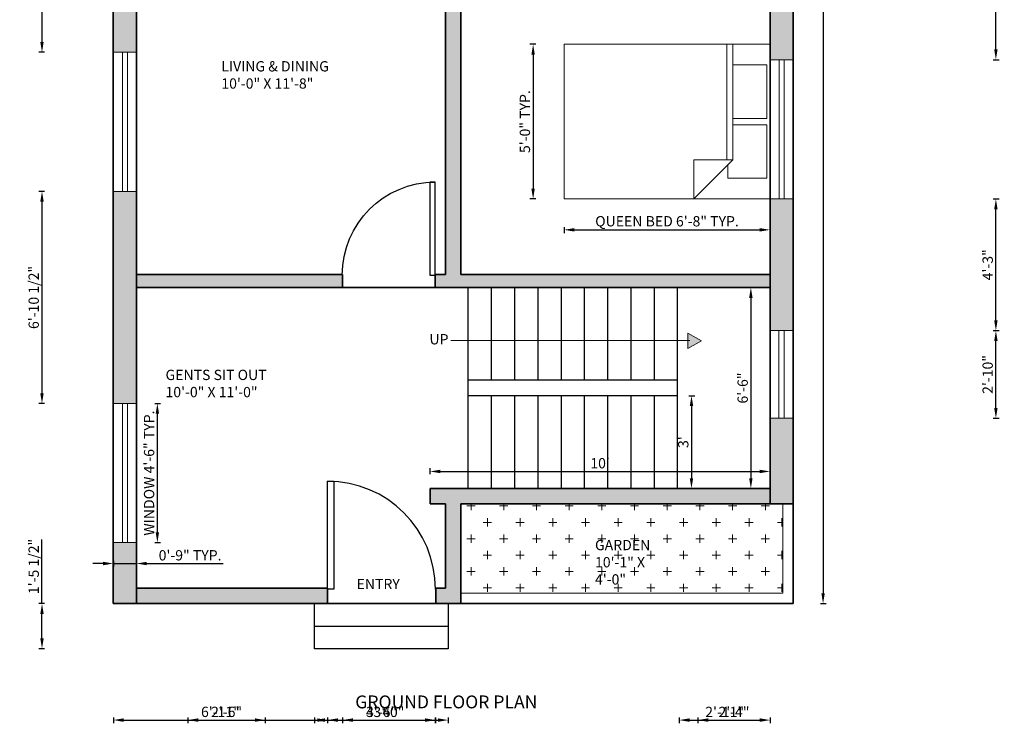
# Model space of a CAD drawing. Units: inches. Extents: x -34 to 348, y -513 to 46.
# Tile 1 of 2: x -34 to 348, y -513 to -240. Entities that reach past the tile are written whole.
import ezdxf

# ---------------------------------------------------------------- set-up
doc = ezdxf.new("R2010")
doc.units = ezdxf.units.IN
for name, color, linetype, lineweight in [('A-ANNO-DIMS', 2, 'Continuous', 18), ('A-ANNO-SYMB', 7, 'Continuous', 18), ('A-ANNO-TEXT', 7, 'Continuous', 18), ('A-AREA-IDEN', 7, 'Continuous', 18), ('A-DOOR', 4, 'Continuous', 25), ('A-FLOR-STRS', 7, 'Continuous', 25), ('A-FURN', 8, 'Continuous', 18), ('A-GLAZ', 6, 'Continuous', 18), ('A-WALL', 7, 'Continuous', 35), ('A-WALL-PATT', 251, 'Continuous', 13), ('L-PLNT', 3, 'Continuous', 18), ('L-PLNT-PATT', 3, 'Continuous', 13)]:
    doc.layers.add(name, color=color, linetype=linetype, lineweight=lineweight)
doc.styles.get("Standard").update_dxf_attribs({"font": 'arial.ttf'})
doc.dimstyles.new('ISO-25', dxfattribs={"dimtxt": 4, "dimasz": 4, "dimexe": 1.25, "dimexo": 0.625, "dimtad": 1, "dimlunit": 3, "dimtxsty": 'Standard', "dimcen": 2.5, "dimadec": 0, "dimazin": 0, "dimtfac": 1, "dimtmove": 0, "dimatfit": 3, "dimfxl": 1, "dimfxlon": 1, "dimarcsym": 0})

# ---------------------------------------------------------------- blocks, each defined once
blk = doc.blocks.new('*U4')
for p, q in [((0, 0), (0, -100)), ((750, 0), (750, -100))]:
    blk.add_line(p, q)
blk.add_lwpolyline([(0, 0), (0, 750), (43.75, 750), (43.75, 0)], close=True)
blk.add_arc((0, 0), 750, 0, 90)
blk = doc.blocks.new('Bed - Queen')
for p, q in [((0, -80.00003), (0, 0)), ((0, 0), (59.99999, 0)), ((59.99999, 0), (59.99999, -80.00003)), ((7.99999, -1.2), (28.79998, -1.2)), ((7.99999, -14.4), (7.99999, -1.2)), ((28.79998, -1.2), (28.79998, -14.4)), ((31.19999, -1.2), (51.99999, -1.2)), ((31.19999, -14.4), (31.19999, -1.2)), ((51.99999, -1.2), (51.99999, -16.4)), ((0, -14.4), (44.8, -14.4)), ((59.99999, -29.6), (44.8, -14.4)), ((44.8, -14.4), (44.8, -29.6)), ((44.8, -16.8), (0, -16.8)), ((51.99999, -16.4), (46.79936, -16.4)), ((44.8, -29.6), (59.99999, -29.6)), ((59.99999, -80.00003), (0, -80.00003))]:
    blk.add_line(p, q)
blk = doc.blocks.new('*D9')
at = {"layer": 'A-ANNO-DIMS', "color": 0, "lineweight": -2, "transparency": 16777216}
for p, q in [((225.63, -385.93), (227.88, -385.93)), ((226.63, -389.93), (226.63, -417.93)), ((225.63, -421.93), (227.88, -421.93))]:
    blk.add_line(p, q, dxfattribs=at)
at = {"layer": 'A-ANNO-DIMS', "color": 0, "transparency": 16777216}
for points in [[(225.96, -389.93), (227.3, -389.93), (226.63, -385.93)], [(225.96, -417.93), (227.3, -417.93), (226.63, -421.93)]]:
    blk.add_solid(points, dxfattribs=at)
at = {"layer": 'Defpoints', "color": 0, "transparency": 16777216}
for p in [(221.13, -385.93), (221.13, -421.93), (226.63, -421.93)]:
    blk.add_point(p, dxfattribs=at)
at = {"layer": 'A-ANNO-DIMS', "color": 0, "transparency": 16777216, "insert": (223.96, -403.93), "char_height": 4, "attachment_point": 5, "rotation": 90}
blk.add_mtext("3'", dxfattribs=at)
blk = doc.blocks.new('*D10')
at = {"layer": 'A-ANNO-DIMS', "color": 0, "lineweight": -2, "transparency": 16777216}
for p, q in [((125.13, -416.3), (125.13, -414.05)), ((129.13, -415.3), (253.13, -415.3)), ((257.13, -416.3), (257.13, -414.05))]:
    blk.add_line(p, q, dxfattribs=at)
at = {"layer": 'A-ANNO-DIMS', "color": 0, "transparency": 16777216}
for points in [[(129.13, -414.64), (129.13, -415.97), (125.13, -415.3)], [(253.13, -414.64), (253.13, -415.97), (257.13, -415.3)]]:
    blk.add_solid(points, dxfattribs=at)
at = {"layer": 'Defpoints', "color": 0, "transparency": 16777216}
for p in [(257.13, -415.3), (125.13, -421.93), (257.13, -421.93)]:
    blk.add_point(p, dxfattribs=at)
at = {"layer": 'A-ANNO-DIMS', "color": 0, "transparency": 16777216, "insert": (191.13, -412.63), "char_height": 4, "attachment_point": 5}
blk.add_mtext("10'", dxfattribs=at)
blk = doc.blocks.new('*D11')
at = {"layer": 'A-ANNO-DIMS', "color": 0, "lineweight": -2, "transparency": 16777216}
for p, q in [((250.69, -343.93), (248.44, -343.93)), ((249.69, -347.93), (249.69, -417.93)), ((250.69, -421.93), (248.44, -421.93))]:
    blk.add_line(p, q, dxfattribs=at)
at = {"layer": 'A-ANNO-DIMS', "color": 0, "transparency": 16777216}
for points in [[(249.02, -347.93), (250.35, -347.93), (249.69, -343.93)], [(249.02, -417.93), (250.35, -417.93), (249.69, -421.93)]]:
    blk.add_solid(points, dxfattribs=at)
at = {"layer": 'Defpoints', "color": 0, "transparency": 16777216}
for p in [(257.13, -343.93), (249.69, -421.93), (257.13, -421.93)]:
    blk.add_point(p, dxfattribs=at)
at = {"layer": 'A-ANNO-DIMS', "color": 0, "transparency": 16777216, "insert": (247.02, -382.93), "char_height": 4, "attachment_point": 5, "rotation": 90}
blk.add_mtext('6\'-6"', dxfattribs=at)
blk = doc.blocks.new('*D13')
at = {"layer": 'A-ANNO-DIMS', "color": 0, "lineweight": -2, "transparency": 16777216}
for p, q in [((276.72, 13.4), (278.97, 13.4)), ((277.72, 9.4), (277.72, -462.6)), ((276.72, -466.6), (278.97, -466.6))]:
    blk.add_line(p, q, dxfattribs=at)
at = {"layer": 'A-ANNO-DIMS', "color": 0, "transparency": 16777216}
for points in [[(277.06, 9.4), (278.39, 9.4), (277.72, 13.4)], [(277.06, -462.6), (278.39, -462.6), (277.72, -466.6)]]:
    blk.add_solid(points, dxfattribs=at)
at = {"layer": 'Defpoints', "color": 0, "transparency": 16777216}
for p in [(266.13, 13.4), (266.13, -466.6), (277.72, -466.6)]:
    blk.add_point(p, dxfattribs=at)
at = {"layer": 'A-ANNO-DIMS', "color": 0, "transparency": 16777216, "insert": (275.05, -226.6), "char_height": 4, "attachment_point": 5, "rotation": 90}
blk.add_mtext("40'", dxfattribs=at)
blk = doc.blocks.new('WIN-54IN')
for p, q in [((3.5, 54), (3.5, 0)), ((5.5, 54), (5.5, 0))]:
    blk.add_line(p, q)
blk.add_lwpolyline([(0, 54), (9, 54), (9, 0), (0, 0)], close=True)
blk = doc.blocks.new('*D16')
at = {"layer": 'A-ANNO-DIMS', "color": 0, "lineweight": -2, "transparency": 16777216}
for p, q in [((18.23, -388.94), (20.48, -388.94)), ((19.23, -438.94), (19.23, -392.94)), ((18.23, -442.94), (20.48, -442.94))]:
    blk.add_line(p, q, dxfattribs=at)
at = {"layer": 'A-ANNO-DIMS', "color": 0, "transparency": 16777216}
for points in [[(18.56, -392.94), (19.89, -392.94), (19.23, -388.94)], [(18.56, -438.94), (19.89, -438.94), (19.23, -442.94)]]:
    blk.add_solid(points, dxfattribs=at)
at = {"layer": 'Defpoints', "color": 0, "transparency": 16777216}
for p in [(11.13, -388.94), (19.23, -388.94), (11.13, -442.94)]:
    blk.add_point(p, dxfattribs=at)
at = {"layer": 'A-ANNO-DIMS', "color": 0, "transparency": 16777216, "insert": (16.53, -415.94), "char_height": 4, "attachment_point": 5, "rotation": 90}
blk.add_mtext('WINDOW 4\'-6" TYP.', dxfattribs=at)
blk = doc.blocks.new('*D17')
at = {"layer": 'A-ANNO-DIMS', "color": 0, "lineweight": -2, "transparency": 16777216}
for p, q in [((-1.87, -451.04), (-5.87, -451.04)), ((2.13, -450.04), (2.13, -452.29)), ((2.13, -451.04), (11.13, -451.04)), ((11.13, -450.04), (11.13, -452.29)), ((15.13, -451.04), (44.76, -451.04))]:
    blk.add_line(p, q, dxfattribs=at)
at = {"layer": 'A-ANNO-DIMS', "color": 0, "transparency": 16777216}
for points in [[(-1.87, -450.37), (-1.87, -451.71), (2.13, -451.04)], [(15.13, -450.37), (15.13, -451.71), (11.13, -451.04)]]:
    blk.add_solid(points, dxfattribs=at)
at = {"layer": 'Defpoints', "color": 0, "transparency": 16777216}
for p in [(2.13, -442.94), (11.13, -442.94), (11.13, -451.04)]:
    blk.add_point(p, dxfattribs=at)
at = {"layer": 'A-ANNO-DIMS', "color": 0, "transparency": 16777216, "insert": (31.94, -448.37), "char_height": 4, "attachment_point": 5}
blk.add_mtext('0\'-9" TYP.', dxfattribs=at)
blk = doc.blocks.new('*D20')
at = {"layer": 'A-ANNO-DIMS', "color": 0, "lineweight": -2, "transparency": 16777216}
for p, q in [((177.13, -320.53), (177.13, -322.78)), ((257.13, -320.53), (257.13, -322.78)), ((181.13, -321.53), (253.13, -321.53))]:
    blk.add_line(p, q, dxfattribs=at)
at = {"layer": 'A-ANNO-DIMS', "color": 0, "transparency": 16777216}
for points in [[(181.13, -320.87), (181.13, -322.2), (177.13, -321.53)], [(253.13, -320.87), (253.13, -322.2), (257.13, -321.53)]]:
    blk.add_solid(points, dxfattribs=at)
at = {"layer": 'Defpoints', "color": 0, "transparency": 16777216}
for p in [(177.13, -309.53), (257.13, -309.53), (257.13, -321.53)]:
    blk.add_point(p, dxfattribs=at)
at = {"layer": 'A-ANNO-DIMS', "color": 0, "transparency": 16777216, "insert": (217.13, -318.72), "char_height": 4, "attachment_point": 5}
blk.add_mtext('QUEEN BED 6\'-8" TYP.', dxfattribs=at)
blk = doc.blocks.new('*D21')
at = {"layer": 'A-ANNO-DIMS', "color": 0, "lineweight": -2, "transparency": 16777216}
for p, q in [((166.13, -249.53), (163.88, -249.53)), ((165.13, -253.53), (165.13, -305.53)), ((166.13, -309.53), (163.88, -309.53))]:
    blk.add_line(p, q, dxfattribs=at)
at = {"layer": 'A-ANNO-DIMS', "color": 0, "transparency": 16777216}
for points in [[(164.46, -253.53), (165.79, -253.53), (165.13, -249.53)], [(164.46, -305.53), (165.79, -305.53), (165.13, -309.53)]]:
    blk.add_solid(points, dxfattribs=at)
at = {"layer": 'Defpoints', "color": 0, "transparency": 16777216}
for p in [(177.13, -249.53), (165.13, -309.53), (177.13, -309.53)]:
    blk.add_point(p, dxfattribs=at)
at = {"layer": 'A-ANNO-DIMS', "color": 0, "transparency": 16777216, "insert": (162.46, -279.53), "char_height": 4, "attachment_point": 5, "rotation": 90}
blk.add_mtext('5\'-0" TYP.', dxfattribs=at)
blk = doc.blocks.new('*D28')
at = {"layer": 'A-ANNO-DIMS', "color": 0, "lineweight": -2, "transparency": 16777216}
for p, q in [((80.3, -510.8), (80.3, -513.05)), ((84.3, -511.8), (128.17, -511.8)), ((132.17, -510.8), (132.17, -513.05))]:
    blk.add_line(p, q, dxfattribs=at)
at = {"layer": 'A-ANNO-DIMS', "color": 0, "transparency": 16777216}
for points in [[(84.3, -511.13), (84.3, -512.47), (80.3, -511.8)], [(128.17, -511.13), (128.17, -512.47), (132.17, -511.8)]]:
    blk.add_solid(points, dxfattribs=at)
at = {"layer": 'Defpoints', "color": 0, "transparency": 16777216}
for p in [(80.3, -484.1), (132.17, -484.1), (132.17, -511.8)]:
    blk.add_point(p, dxfattribs=at)
at = {"layer": 'A-ANNO-DIMS', "color": 0, "transparency": 16777216, "insert": (106.23, -509.17), "char_height": 4, "attachment_point": 5}
blk.add_mtext('4\'-4"', dxfattribs=at)
blk = doc.blocks.new('*D29')
at = {"layer": 'A-ANNO-DIMS', "color": 0, "lineweight": -2, "transparency": 16777216}
for p, q in [((-25.57, -466.6), (-25.57, -441.77)), ((-24.57, -466.6), (-26.82, -466.6)), ((-25.57, -480.1), (-25.57, -470.6)), ((-24.57, -484.1), (-26.82, -484.1))]:
    blk.add_line(p, q, dxfattribs=at)
at = {"layer": 'A-ANNO-DIMS', "color": 0, "transparency": 16777216}
for points in [[(-26.24, -470.6), (-24.91, -470.6), (-25.57, -466.6)], [(-26.24, -480.1), (-24.91, -480.1), (-25.57, -484.1)]]:
    blk.add_solid(points, dxfattribs=at)
at = {"layer": 'Defpoints', "color": 0, "transparency": 16777216}
for p in [(-25.57, -466.6), (80.3, -466.6), (80.3, -484.1)]:
    blk.add_point(p, dxfattribs=at)
at = {"layer": 'A-ANNO-DIMS', "color": 0, "transparency": 16777216, "insert": (-28.27, -452.18), "char_height": 4, "attachment_point": 5, "rotation": 90}
blk.add_mtext('1\'-5 1/2"', dxfattribs=at)
blk = doc.blocks.new('*D30')
at = {"layer": 'A-ANNO-DIMS', "color": 0, "lineweight": -2, "transparency": 16777216}
for p, q in [((85.32, -510.8), (85.32, -513.05)), ((89.32, -511.8), (123.24, -511.8)), ((127.24, -510.8), (127.24, -513.05))]:
    blk.add_line(p, q, dxfattribs=at)
at = {"layer": 'A-ANNO-DIMS', "color": 0, "transparency": 16777216}
for points in [[(89.32, -511.13), (89.32, -512.47), (85.32, -511.8)], [(123.24, -511.13), (123.24, -512.47), (127.24, -511.8)]]:
    blk.add_solid(points, dxfattribs=at)
at = {"layer": 'Defpoints', "color": 0, "transparency": 16777216}
for p in [(85.32, -466.6), (127.24, -466.6), (127.24, -511.8)]:
    blk.add_point(p, dxfattribs=at)
at = {"layer": 'A-ANNO-DIMS', "color": 0, "transparency": 16777216, "insert": (106.28, -509.13), "char_height": 4, "attachment_point": 5}
blk.add_mtext('3\'-6"', dxfattribs=at)
blk = doc.blocks.new('*D31')
at = {"layer": 'A-ANNO-DIMS', "color": 0, "lineweight": -2, "transparency": 16777216}
for p, q in [((2.13, -510.8), (2.13, -513.05)), ((6.13, -511.8), (81.32, -511.8)), ((85.32, -510.8), (85.32, -513.05))]:
    blk.add_line(p, q, dxfattribs=at)
at = {"layer": 'A-ANNO-DIMS', "color": 0, "transparency": 16777216}
for points in [[(6.13, -511.13), (6.13, -512.47), (2.13, -511.8)], [(81.32, -511.13), (81.32, -512.47), (85.32, -511.8)]]:
    blk.add_solid(points, dxfattribs=at)
at = {"layer": 'Defpoints', "color": 0, "transparency": 16777216}
for p in [(2.13, -466.6), (85.32, -466.6), (85.32, -511.8)]:
    blk.add_point(p, dxfattribs=at)
at = {"layer": 'A-ANNO-DIMS', "color": 0, "transparency": 16777216, "insert": (43.72, -509.13), "char_height": 4, "attachment_point": 5}
blk.add_mtext('6\'-11"', dxfattribs=at)
blk = doc.blocks.new('*D32')
at = {"layer": 'A-ANNO-DIMS', "color": 0, "lineweight": -2, "transparency": 16777216}
for p, q in [((91.13, -510.8), (91.13, -513.05)), ((95.13, -511.8), (123.13, -511.8)), ((127.13, -510.8), (127.13, -513.05))]:
    blk.add_line(p, q, dxfattribs=at)
at = {"layer": 'A-ANNO-DIMS', "color": 0, "transparency": 16777216}
for points in [[(95.13, -511.13), (95.13, -512.47), (91.13, -511.8)], [(123.13, -511.13), (123.13, -512.47), (127.13, -511.8)]]:
    blk.add_solid(points, dxfattribs=at)
at = {"layer": 'Defpoints', "color": 0, "transparency": 16777216}
for p in [(91.13, -343.93), (127.13, -343.93), (127.13, -511.8)]:
    blk.add_point(p, dxfattribs=at)
at = {"layer": 'A-ANNO-DIMS', "color": 0, "transparency": 16777216, "insert": (109.13, -509.13), "char_height": 4, "attachment_point": 5}
blk.add_mtext('3\'-0"', dxfattribs=at)
blk = doc.blocks.new('*D33')
at = {"layer": 'A-ANNO-DIMS', "color": 0, "lineweight": -2, "transparency": 16777216}
for p, q in [((31.1, -510.8), (31.1, -513.05)), ((35.1, -511.8), (57.12, -511.8)), ((61.12, -510.8), (61.12, -513.05))]:
    blk.add_line(p, q, dxfattribs=at)
at = {"layer": 'A-ANNO-DIMS', "color": 0, "transparency": 16777216}
for points in [[(35.1, -511.13), (35.1, -512.47), (31.1, -511.8)], [(57.12, -511.13), (57.12, -512.47), (61.12, -511.8)]]:
    blk.add_solid(points, dxfattribs=at)
at = {"layer": 'Defpoints', "color": 0, "transparency": 16777216}
for p in [(31.1, -137.74), (61.12, -137.74), (61.12, -511.8)]:
    blk.add_point(p, dxfattribs=at)
at = {"layer": 'A-ANNO-DIMS', "color": 0, "transparency": 16777216, "insert": (46.11, -509.13), "char_height": 4, "attachment_point": 5}
blk.add_mtext('2\'-6"', dxfattribs=at)
blk = doc.blocks.new('*D41')
at = {"layer": 'A-ANNO-DIMS', "color": 0, "lineweight": -2, "transparency": 16777216}
for p, q in [((-24.57, -190.01), (-26.82, -190.01)), ((-25.57, -194.01), (-25.57, -248.61)), ((-24.57, -252.61), (-26.82, -252.61))]:
    blk.add_line(p, q, dxfattribs=at)
at = {"layer": 'A-ANNO-DIMS', "color": 0, "transparency": 16777216}
for points in [[(-26.24, -194.01), (-24.91, -194.01), (-25.57, -190.01)], [(-26.24, -248.61), (-24.91, -248.61), (-25.57, -252.61)]]:
    blk.add_solid(points, dxfattribs=at)
at = {"layer": 'Defpoints', "color": 0, "transparency": 16777216}
for p in [(2.13, -190.01), (-25.57, -252.61), (2.13, -252.61)]:
    blk.add_point(p, dxfattribs=at)
at = {"layer": 'A-ANNO-DIMS', "color": 0, "transparency": 16777216, "insert": (-28.27, -221.31), "char_height": 4, "attachment_point": 5, "rotation": 90}
blk.add_mtext('5\'-2 1/2"', dxfattribs=at)
blk = doc.blocks.new('*D42')
at = {"layer": 'A-ANNO-DIMS', "color": 0, "lineweight": -2, "transparency": 16777216}
for p, q in [((-24.57, -306.61), (-26.82, -306.61)), ((-25.57, -310.61), (-25.57, -384.94)), ((-24.57, -388.94), (-26.82, -388.94))]:
    blk.add_line(p, q, dxfattribs=at)
at = {"layer": 'A-ANNO-DIMS', "color": 0, "transparency": 16777216}
for points in [[(-26.24, -310.61), (-24.91, -310.61), (-25.57, -306.61)], [(-26.24, -384.94), (-24.91, -384.94), (-25.57, -388.94)]]:
    blk.add_solid(points, dxfattribs=at)
at = {"layer": 'Defpoints', "color": 0, "transparency": 16777216}
for p in [(2.13, -306.61), (-25.57, -388.94), (2.13, -388.94)]:
    blk.add_point(p, dxfattribs=at)
at = {"layer": 'A-ANNO-DIMS', "color": 0, "transparency": 16777216, "insert": (-28.27, -347.78), "char_height": 4, "attachment_point": 5, "rotation": 90}
blk.add_mtext('6\'-10 1/2"', dxfattribs=at)
blk = doc.blocks.new('*D45')
at = {"layer": 'A-ANNO-DIMS', "color": 0, "lineweight": -2, "transparency": 16777216}
for p, q in [((343.83, -190.01), (346.08, -190.01)), ((344.83, -251.53), (344.83, -194.01)), ((343.83, -255.53), (346.08, -255.53))]:
    blk.add_line(p, q, dxfattribs=at)
at = {"layer": 'A-ANNO-DIMS', "color": 0, "transparency": 16777216}
for points in [[(344.16, -194.01), (345.49, -194.01), (344.83, -190.01)], [(344.16, -251.53), (345.49, -251.53), (344.83, -255.53)]]:
    blk.add_solid(points, dxfattribs=at)
at = {"layer": 'Defpoints', "color": 0, "transparency": 16777216}
for p in [(266.13, -190.01), (344.83, -190.01), (266.13, -255.53)]:
    blk.add_point(p, dxfattribs=at)
at = {"layer": 'A-ANNO-DIMS', "color": 0, "transparency": 16777216, "insert": (342.13, -222.77), "char_height": 4, "attachment_point": 5, "rotation": 90}
blk.add_mtext('5\'-5 1/2"', dxfattribs=at)
blk = doc.blocks.new('*D46')
at = {"layer": 'A-ANNO-DIMS', "color": 0, "lineweight": -2, "transparency": 16777216}
for p, q in [((343.83, -309.53), (346.08, -309.53)), ((344.83, -356.66), (344.83, -313.53)), ((343.83, -360.66), (346.08, -360.66))]:
    blk.add_line(p, q, dxfattribs=at)
at = {"layer": 'A-ANNO-DIMS', "color": 0, "transparency": 16777216}
for points in [[(344.16, -313.53), (345.49, -313.53), (344.83, -309.53)], [(344.16, -356.66), (345.49, -356.66), (344.83, -360.66)]]:
    blk.add_solid(points, dxfattribs=at)
at = {"layer": 'Defpoints', "color": 0, "transparency": 16777216}
for p in [(266.13, -309.53), (344.83, -309.53), (266.11, -360.66)]:
    blk.add_point(p, dxfattribs=at)
at = {"layer": 'A-ANNO-DIMS', "color": 0, "transparency": 16777216, "insert": (342.16, -335.1), "char_height": 4, "attachment_point": 5, "rotation": 90}
blk.add_mtext('4\'-3"', dxfattribs=at)
blk = doc.blocks.new('*D47')
at = {"layer": 'A-ANNO-DIMS', "color": 0, "lineweight": -2, "transparency": 16777216}
for p, q in [((343.83, -360.66), (346.08, -360.66)), ((344.83, -390.66), (344.83, -364.66)), ((343.83, -394.66), (346.08, -394.66))]:
    blk.add_line(p, q, dxfattribs=at)
at = {"layer": 'A-ANNO-DIMS', "color": 0, "transparency": 16777216}
for points in [[(344.16, -364.66), (345.49, -364.66), (344.83, -360.66)], [(344.16, -390.66), (345.49, -390.66), (344.83, -394.66)]]:
    blk.add_solid(points, dxfattribs=at)
at = {"layer": 'Defpoints', "color": 0, "transparency": 16777216}
for p in [(266.11, -360.66), (344.83, -360.66), (266.11, -394.66)]:
    blk.add_point(p, dxfattribs=at)
at = {"layer": 'A-ANNO-DIMS', "color": 0, "transparency": 16777216, "insert": (342.16, -377.66), "char_height": 4, "attachment_point": 5, "rotation": 90}
blk.add_mtext('2\'-10"', dxfattribs=at)
blk = doc.blocks.new('*D49')
at = {"layer": 'A-ANNO-DIMS', "color": 0, "lineweight": -2, "transparency": 16777216}
for p, q in [((229.13, -510.8), (229.13, -513.05)), ((233.13, -511.8), (253.13, -511.8)), ((257.13, -510.8), (257.13, -513.05))]:
    blk.add_line(p, q, dxfattribs=at)
at = {"layer": 'A-ANNO-DIMS', "color": 0, "transparency": 16777216}
for points in [[(233.13, -511.13), (233.13, -512.47), (229.13, -511.8)], [(253.13, -511.13), (253.13, -512.47), (257.13, -511.8)]]:
    blk.add_solid(points, dxfattribs=at)
at = {"layer": 'Defpoints', "color": 0, "transparency": 16777216}
for p in [(229.13, -167.74), (257.13, -178.24), (257.13, -511.8)]:
    blk.add_point(p, dxfattribs=at)
at = {"layer": 'A-ANNO-DIMS', "color": 0, "transparency": 16777216, "insert": (243.13, -509.17), "char_height": 4, "attachment_point": 5}
blk.add_mtext('2\'-4"', dxfattribs=at)
blk = doc.blocks.new('*D50')
at = {"layer": 'A-ANNO-DIMS', "color": 0, "lineweight": -2, "transparency": 16777216}
for p, q in [((221.89, -510.8), (221.89, -513.05)), ((225.89, -511.8), (253.13, -511.8)), ((257.13, -510.8), (257.13, -513.05))]:
    blk.add_line(p, q, dxfattribs=at)
at = {"layer": 'A-ANNO-DIMS', "color": 0, "transparency": 16777216}
for points in [[(225.89, -511.13), (225.89, -512.47), (221.89, -511.8)], [(253.13, -511.13), (253.13, -512.47), (257.13, -511.8)]]:
    blk.add_solid(points, dxfattribs=at)
at = {"layer": 'Defpoints', "color": 0, "transparency": 16777216}
for p in [(221.89, 4.4), (257.13, 4.4), (257.13, -511.8)]:
    blk.add_point(p, dxfattribs=at)
at = {"layer": 'A-ANNO-DIMS', "color": 0, "transparency": 16777216, "insert": (239.51, -509.17), "char_height": 4, "attachment_point": 5}
blk.add_mtext('2\'-11"', dxfattribs=at)
blk = doc.blocks.new('*D51')
at = {"layer": 'A-ANNO-DIMS', "color": 0, "lineweight": -2, "transparency": 16777216}
for p, q in [((221.13, 40.1), (221.13, 42.35)), ((257.13, 40.1), (257.13, 42.35)), ((225.13, 41.1), (253.13, 41.1))]:
    blk.add_line(p, q, dxfattribs=at)
at = {"layer": 'A-ANNO-DIMS', "color": 0, "transparency": 16777216}
for points in [[(225.13, 41.77), (225.13, 40.44), (221.13, 41.1)], [(253.13, 41.77), (253.13, 40.44), (257.13, 41.1)]]:
    blk.add_solid(points, dxfattribs=at)
at = {"layer": 'Defpoints', "color": 0, "transparency": 16777216}
for p in [(257.13, 41.1), (221.13, -343.93), (257.13, -343.93)]:
    blk.add_point(p, dxfattribs=at)
at = {"layer": 'A-ANNO-DIMS', "color": 0, "transparency": 16777216, "insert": (239.13, 43.77), "char_height": 4, "attachment_point": 5}
blk.add_mtext('3\'-0"', dxfattribs=at)
blk = doc.blocks.new('*D53')
at = {"layer": 'A-ANNO-DIMS', "color": 0, "lineweight": -2, "transparency": 16777216}
for p, q in [((212.09, 40.1), (212.09, 42.35)), ((221.13, 40.1), (221.13, 42.35)), ((208.09, 41.1), (204.09, 41.1)), ((212.09, 41.1), (221.13, 41.1)), ((225.13, 41.1), (241.01, 41.1))]:
    blk.add_line(p, q, dxfattribs=at)
at = {"layer": 'A-ANNO-DIMS', "color": 0, "transparency": 16777216}
for points in [[(208.09, 41.77), (208.09, 40.44), (212.09, 41.1)], [(225.13, 41.77), (225.13, 40.44), (221.13, 41.1)]]:
    blk.add_solid(points, dxfattribs=at)
at = {"layer": 'Defpoints', "color": 0, "transparency": 16777216}
for p in [(221.13, 41.1), (212.09, -343.93), (221.13, -343.93)]:
    blk.add_point(p, dxfattribs=at)
at = {"layer": 'A-ANNO-DIMS', "color": 0, "transparency": 16777216, "insert": (235.07, 43.77), "char_height": 4, "attachment_point": 5}
blk.add_mtext('0\'-9"', dxfattribs=at)

msp = doc.modelspace()

# ---------------------------------------------------------------- hatches: boundary and pattern name
at = {"layer": 'A-ANNO-SYMB'}
h = msp.add_hatch(color=256, dxfattribs=at)
h.dxf.hatch_style = 1
h.paths.add_polyline_path([(225.262, -361.599), (225.262, -367.599), (230.46, -364.602)])
at = {"layer": 'A-WALL-PATT'}
h = msp.add_hatch(color=256, dxfattribs=at)
h.dxf.hatch_style = 1
h.paths.add_polyline_path([(109.341, 13.405), (2.127, 13.405), (2.127, -25.971), (11.127, -25.971), (11.127, 4.405), (109.341, 4.405)])
h.paths.add_polyline_path([(266.127, 13.405), (127.341, 13.405), (127.341, 4.405), (131.127, 4.405), (137.127, 4.405), (257.127, 4.405), (257.127, -24.182), (266.127, -24.182)])
h.paths.add_polyline_path([(11.127, -79.971), (2.127, -79.971), (2.127, -172.013), (11.127, -172.013)])
h.paths.add_polyline_path([(65.127, -127.595), (11.127, -127.595), (11.127, -133.595), (59.127, -133.595), (59.127, -137.743), (61.124, -137.743), (65.127, -137.743), (65.127, -133.595)])
h.paths.add_polyline_path([(65.127, -167.764), (61.124, -167.764, -0.0092932), (60.008, -167.743), (59.127, -167.743), (59.127, -193.595), (11.127, -193.595), (11.127, -199.595), (59.127, -199.595), (65.127, -199.595)])
h.paths.add_polyline_path([(11.127, -190.013), (2.127, -190.013), (2.127, -252.614), (11.127, -252.614)])
h.paths.add_polyline_path([(11.127, -306.614), (2.127, -306.614), (2.127, -388.939), (11.127, -388.939)])
h.paths.add_polyline_path([(85.316, -461.006), (85.316, -460.595), (11.127, -460.595), (11.127, -466.595), (85.316, -466.595)])
h.paths.add_polyline_path([(11.127, -442.939), (2.127, -442.939), (2.127, -466.595), (11.127, -466.595)])
h.paths.add_polyline_path([(137.127, -427.93), (257.127, -427.93), (257.127, -421.93), (131.127, -421.93), (125.127, -421.93), (125.127, -427.93), (131.127, -427.93), (131.127, -460.595), (127.316, -460.595), (127.316, -466.595), (132.166, -466.595), (137.127, -466.595)])
h.paths.add_polyline_path([(266.127, -394.659), (257.127, -394.659), (257.127, -421.93), (257.127, -427.93), (266.127, -427.93)])
h.paths.add_polyline_path([(266.127, -309.532), (257.127, -309.532), (257.127, -343.93), (257.127, -360.659), (266.127, -360.659)])
h.paths.add_polyline_path([(257.127, -338.93), (137.127, -338.93), (137.127, -199.595), (141.127, -199.595), (141.127, -193.595), (131.127, -193.595), (131.127, -338.93), (127.127, -338.93), (127.127, -339.114), (127.127, -343.93), (137.127, -343.93), (257.127, -343.93)])
h.paths.add_polyline_path([(91.006, -338.93), (11.127, -338.93), (11.127, -343.93), (91.006, -343.93)])
h.paths.add_polyline_path([(266.127, -190.013), (257.127, -190.013), (257.127, -255.532), (266.127, -255.532)])
h.paths.add_polyline_path([(257.127, -193.595), (185.127, -193.595), (185.127, -167.989), (179.127, -167.989), (179.127, -193.595), (177.136, -193.595), (177.136, -198.391, -0.0057168), (177.127, -199.214), (177.127, -199.595), (179.127, -199.595), (185.127, -199.595), (257.127, -199.595)])
h.paths.add_polyline_path([(266.127, -78.182), (257.127, -78.182), (257.127, -172.013), (266.127, -172.013)])
h.paths.add_polyline_path([(257.127, -127.595), (177.127, -127.595), (177.127, -133.595), (179.127, -133.595), (179.127, -137.989), (183.118, -137.989), (185.127, -137.989), (185.127, -133.595), (257.127, -133.595)])
h.paths.add_polyline_path([(137.127, 4.405), (131.127, 4.405), (131.127, -127.595), (127.127, -127.595), (127.127, -133.595), (131.127, -133.595), (137.127, -133.595), (141.127, -133.595), (141.127, -128.797), (141.127, -127.595), (137.127, -127.595)])
at = {"layer": 'L-PLNT-PATT'}
h = msp.add_hatch(dxfattribs=at)
h.set_pattern_fill('CROSS', color=256)
h.set_pattern_definition([(0, (-419.374, -35.0104), (6.35, 6.35), [3.175, -9.525]), (90, (-417.7867, -36.598), (-6.35, 6.35), [3.175, -9.525])])
h.paths.add_polyline_path([(262.127, -427.93), (137.127, -427.93), (137.127, -462.595), (262.127, -462.595)])

# ---------------------------------------------------------------- linework, layer by layer
at = {"layer": 'A-ANNO-SYMB'}
msp.add_line((133.139, -364.529), (226.006, -364.529), dxfattribs=at)
msp.add_lwpolyline([(225.262, -361.599), (225.262, -367.599), (230.46, -364.602)], close=True, dxfattribs=at)
at = {"layer": 'A-FLOR-STRS'}
for p, q in [((139.832, -343.93), (139.832, -421.93)), ((139.832, -343.93), (139.832, -379.93)), ((148.865, -343.93), (148.865, -379.93)), ((157.897, -343.93), (157.897, -379.93)), ((166.93, -343.93), (166.93, -379.93)), ((175.963, -343.93), (175.963, -379.93)), ((184.996, -343.93), (184.996, -379.93)), ((194.028, -343.93), (194.028, -379.93)), ((203.061, -343.93), (203.061, -379.93)), ((212.094, -343.93), (212.094, -379.93)), ((221.127, -343.93), (221.127, -379.93)), ((221.127, -379.93), (139.832, -379.93)), ((221.127, -379.93), (221.127, -385.93)), ((221.127, -385.93), (139.832, -385.93)), ((139.832, -385.93), (139.832, -421.93)), ((148.865, -385.93), (148.865, -421.93)), ((157.897, -385.93), (157.897, -421.93)), ((166.93, -385.93), (166.93, -421.93)), ((175.963, -385.93), (175.963, -421.93)), ((184.996, -385.93), (184.996, -421.93)), ((194.028, -385.93), (194.028, -421.93)), ((203.061, -385.93), (203.061, -421.93)), ((212.094, -385.93), (212.094, -421.93)), ((221.127, -385.93), (221.127, -421.93)), ((80.303, -475.348), (132.166, -475.348))]:
    msp.add_line(p, q, dxfattribs=at)
msp.add_lwpolyline([(80.303, -466.595), (132.166, -466.595), (132.166, -484.1), (80.303, -484.1)], close=True, dxfattribs=at)
at = {"layer": 'A-GLAZ'}
for p, q in [((5.627, -252.614), (5.627, -306.614)), ((7.627, -252.614), (7.627, -306.614)), ((260.606, -360.659), (260.606, -394.659)), ((262.606, -360.659), (262.606, -394.659))]:
    msp.add_line(p, q, dxfattribs=at)
for points in [[(2.127, -252.614), (11.127, -252.614), (11.127, -306.614), (2.127, -306.614)], [(257.106, -360.659), (266.106, -360.659), (266.106, -394.659), (257.106, -394.659)]]:
    msp.add_lwpolyline(points, close=True, dxfattribs=at)
at = {"layer": 'A-WALL'}
for p, q in [((2.127, -466.595), (2.127, 13.405)), ((266.127, 13.405), (266.127, -427.93)), ((11.127, -466.595), (11.127, 4.405)), ((257.127, 4.405), (257.127, -343.93)), ((131.127, -338.93), (131.127, -193.595)), ((137.127, -338.93), (137.127, -199.595)), ((91.127, -338.93), (11.127, -338.93)), ((91.127, -338.93), (91.127, -343.93)), ((131.127, -338.93), (127.127, -338.93)), ((127.127, -338.93), (127.127, -343.93)), ((257.127, -338.93), (137.127, -338.93)), ((137.127, -343.93), (11.127, -343.93)), ((257.127, -343.93), (137.127, -343.93)), ((257.127, -343.93), (257.127, -421.93)), ((131.127, -421.93), (125.127, -421.93)), ((125.127, -421.93), (125.127, -427.93)), ((257.127, -421.93), (131.127, -421.93)), ((257.127, -421.93), (257.127, -427.93)), ((125.127, -427.93), (131.127, -427.93)), ((131.127, -460.595), (131.127, -427.93)), ((137.127, -466.595), (137.127, -427.93)), ((266.127, -427.93), (137.127, -427.93)), ((266.127, -427.93), (266.127, -466.595)), ((85.316, -460.595), (11.127, -460.595)), ((85.316, -460.595), (85.316, -466.595)), ((131.127, -460.595), (127.316, -460.595)), ((127.316, -460.595), (127.316, -466.595)), ((11.127, -466.595), (2.127, -466.595)), ((131.127, -466.595), (11.127, -466.595)), ((266.127, -466.595), (131.127, -466.595))]:
    msp.add_line(p, q, dxfattribs=at)
at = {"layer": 'L-PLNT'}
for p, q in [((262.127, -427.93), (262.127, -462.595)), ((262.127, -462.595), (137.127, -462.595))]:
    msp.add_line(p, q, dxfattribs=at)

# ---------------------------------------------------------------- block references
at = {"layer": 'A-DOOR'}
for p, xscale, yscale, zscale in [((127.127, -339.114), -0.0481608788298955, 0.0481608788298955, 0.0481608788298955), ((85.316, -461.006), 0.0558927172393197, 0.0558927172393197, 0.0558927172393197)]:
    msp.add_blockref('*U4', p, dxfattribs=dict(at, xscale=xscale, yscale=yscale, zscale=zscale))
at = {"layer": 'A-FURN', "rotation": 270}
msp.add_blockref('Bed - Queen', (257.127, -249.532), dxfattribs=at)
at = {"layer": 'A-GLAZ'}
for p in [(257.127, -309.532), (2.127, -442.939)]:
    msp.add_blockref('WIN-54IN', p, dxfattribs=at)

# ---------------------------------------------------------------- texts
at = {"layer": 'A-ANNO-TEXT', "attachment_point": 1}
for s, width, insert, char_height in [('UP', 6.65188, (124.876, -361.99), 4), ('ENTRY', 18.17772, (96.586, -456.992), 4), ('GROUND FLOOR PLAN', 117.68355, (96.068, -502.254), 5)]:
    msp.add_mtext_dynamic_manual_height_columns(s, width=width, gutter_width=12.5, heights=[0], dxfattribs=dict(at, insert=insert, char_height=char_height))
at = {"layer": 'A-AREA-IDEN', "char_height": 4, "attachment_point": 1}
for s, width, insert in [('LIVING & DINING\\P10\'-0" X 11\'-8"', 84.85633, (44.067, -256.069)), ('GENTS SIT OUT\\P10\'-0" X 11\'-0"', 73.26556, (22.393, -375.834)), ('GARDEN\\P10\'-1" X 4\'-0"', 31.86664, (189.162, -441.871))]:
    msp.add_mtext_dynamic_manual_height_columns(s, width=width, gutter_width=12.5, heights=[0], dxfattribs=dict(at, insert=insert))

# ---------------------------------------------------------------- dimensions: what is measured, and where the dimension line sits
at = {"layer": 'A-ANNO-DIMS'}
for base, p1, p2, picture, middle in [((221.127, 41.105), (212.094, -343.93), (221.127, -343.93), '*D53', (235.068, 43.772)), ((257.127, 41.105), (221.127, -343.93), (257.127, -343.93), '*D51', (239.127, 43.773)), ((257.127, -511.8), (221.891, 4.405), (257.127, 4.405), '*D50', (239.509, -509.166)), ((61.124, -511.8), (31.103, -137.743), (61.124, -137.743), '*D33', (46.114, -509.132)), ((257.127, -511.8), (229.127, -167.738), (257.127, -178.238), '*D49', (243.127, -509.166)), ((127.127, -511.8), (91.127, -343.93), (127.127, -343.93), '*D32', (109.127, -509.131)), ((85.316, -511.8), (2.127, -466.595), (85.316, -466.595), '*D31', (43.721, -509.132)), ((127.235, -511.8), (85.316, -466.595), (127.235, -466.595), '*D30', (106.276, -509.131)), ((132.166, -511.8), (80.303, -484.1), (132.166, -484.1), '*D28', (106.235, -509.175))]:
    dim = msp.add_linear_dim(base=base, p1=p1, p2=p2, dimstyle='ISO-25', override={"dimdec": 1, "dimlfac": 1, "dimrnd": 0, "dimzin": 1, "dimdsep": 46, "dimlunit": 4, "dimfrac": 2}, dxfattribs=at)
    dim.commit()
    dim.dimension.update_dxf_attribs({"geometry": picture, "text_midpoint": middle})
dim = msp.add_linear_dim(base=(277.722, -466.595), p1=(266.127, 13.405), p2=(266.127, -466.595), angle=90, dimstyle='ISO-25', override={"dimclrd": 0, "dimclre": 0, "dimclrt": 0}, dxfattribs=at)
dim.commit()
dim.dimension.update_dxf_attribs({"geometry": '*D13', "text_midpoint": (277.722, -226.595), "dimtype": 160})
for base, p1, p2, override, picture, middle in [((-25.573, -252.614), (2.127, -190.013), (2.127, -252.614), {"dimdec": 1, "dimlfac": 1, "dimrnd": 0, "dimzin": 1, "dimdsep": 46, "dimlunit": 4, "dimfrac": 2}, '*D41', (-28.266, -221.313)), ((344.827, -190.013), (266.127, -255.532), (266.127, -190.013), {"dimdec": 1, "dimlfac": 1, "dimrnd": 0, "dimzin": 1, "dimdsep": 46, "dimlunit": 4, "dimfrac": 2}, '*D45', (342.134, -222.772)), ((-25.573, -388.939), (2.127, -306.614), (2.127, -388.939), {"dimdec": 1, "dimlfac": 1, "dimrnd": 0, "dimzin": 1, "dimdsep": 46, "dimlunit": 4, "dimfrac": 2}, '*D42', (-28.266, -347.776)), ((344.827, -309.532), (266.106, -360.659), (266.127, -309.532), {"dimdec": 1, "dimlfac": 1, "dimrnd": 0, "dimzin": 1, "dimdsep": 46, "dimlunit": 4, "dimfrac": 2}, '*D46', (342.158, -335.095)), ((249.687, -421.93), (257.127, -343.93), (257.127, -421.93), {"dimclrd": 0, "dimclre": 0, "dimclrt": 0}, '*D11', (247.02, -382.93)), ((344.827, -360.659), (266.106, -394.659), (266.106, -360.659), {"dimdec": 1, "dimlfac": 1, "dimrnd": 0, "dimzin": 1, "dimdsep": 46, "dimlunit": 4, "dimfrac": 2}, '*D47', (342.159, -377.659)), ((226.632, -421.93), (221.127, -385.93), (221.127, -421.93), {"dimclrd": 0, "dimclre": 0, "dimclrt": 0}, '*D9', (223.963, -403.93)), ((-25.573, -466.595), (80.303, -484.1), (80.303, -466.595), {"dimdec": 1, "dimlfac": 1, "dimrnd": 0, "dimzin": 1, "dimdsep": 46, "dimlunit": 4, "dimfrac": 2}, '*D29', (-28.266, -452.182))]:
    dim = msp.add_linear_dim(base=base, p1=p1, p2=p2, angle=90, dimstyle='ISO-25', override=override, dxfattribs=at)
    dim.commit()
    dim.dimension.update_dxf_attribs({"geometry": picture, "text_midpoint": middle})
for base, p1, p2, angle, text, picture, middle in [((165.127, -309.532), (177.127, -249.532), (177.127, -309.532), 270, '<> TYP.', '*D21', (162.459, -279.532)), ((19.227, -388.939), (11.127, -442.939), (11.127, -388.939), 90, 'WINDOW <> TYP.', '*D16', (16.532, -415.939))]:
    dim = msp.add_linear_dim(base=base, p1=p1, p2=p2, angle=angle, text=text, dimstyle='ISO-25', override={"dimdec": 1, "dimlfac": 1, "dimrnd": 0, "dimzin": 1, "dimdsep": 46, "dimlunit": 4, "dimfrac": 2}, dxfattribs=at)
    dim.commit()
    dim.dimension.update_dxf_attribs({"geometry": picture, "text_midpoint": middle})
for base, p1, p2, text, override, picture, middle in [((257.127, -321.532), (177.127, -309.532), (257.127, -309.532), 'QUEEN BED <> TYP.', {"dimdec": 1, "dimlfac": 1, "dimrnd": 0, "dimzin": 1, "dimdsep": 46, "dimlunit": 4, "dimfrac": 2}, '*D20', (217.127, -318.716)), ((257.127, -415.302), (125.127, -421.93), (257.127, -421.93), "10'", {"dimclrd": 0, "dimclre": 0, "dimclrt": 0}, '*D10', (191.127, -412.635)), ((11.127, -451.039), (2.127, -442.939), (11.127, -442.939), '<> TYP.', {"dimdec": 1, "dimlfac": 1, "dimrnd": 0, "dimzin": 1, "dimdsep": 46, "dimlunit": 4, "dimfrac": 2}, '*D17', (31.943, -448.372))]:
    dim = msp.add_linear_dim(base=base, p1=p1, p2=p2, text=text, dimstyle='ISO-25', override=override, dxfattribs=at)
    dim.commit()
    dim.dimension.update_dxf_attribs({"geometry": picture, "text_midpoint": middle})

doc.saveas('drawing.dxf')
